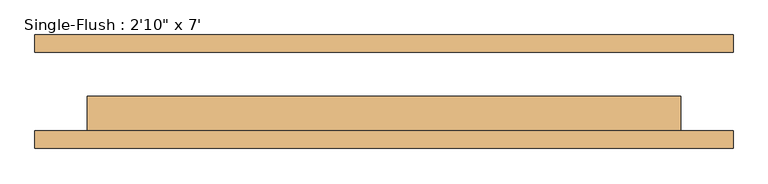
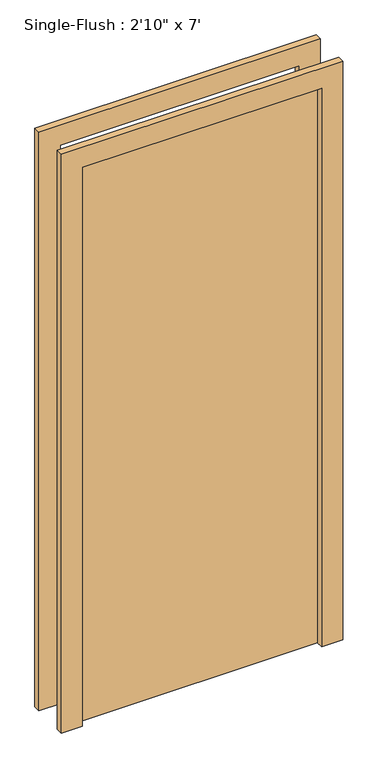
"""IFC4 building model written with IfcOpenShell, lengths in millimetres: door geometry."""

from ifc_helpers import new_model, si_unit, frame, origin, origin_with_axes, place, context, project, spatial, polyline, outline, extrude, source, transform, mapped, element, save


def door_700d3439(model_context):
    return source(origin(), model_context, "Body", "SweptSolid", [
        extrude(outline(polyline([(2209.8, -508.0), (0.0, -508.0), (0.0, -431.8), (2133.6, -431.8), (2133.6, 431.8), (0.0, 431.8), (0.0, 508.0), (2209.8, 508.0), (2209.8, -508.0)])), frame((0.0, -82.55, 0.0), z_axis=(0.0, 1.0, 0.0), x_axis=(0.0, 0.0, 1.0)), (0.0, 0.0, 1.0), 25.4),
        extrude(outline(polyline([(2209.8, 508.0), (2209.8, -508.0), (0.0, -508.0), (0.0, -431.8), (2133.6, -431.8), (2133.6, 431.8), (0.0, 431.8), (0.0, 508.0), (2209.8, 508.0)])), frame((0.0, 57.15, 0.0), z_axis=(0.0, 1.0, 0.0), x_axis=(0.0, 0.0, 1.0)), (0.0, 0.0, 1.0), 25.4),
        extrude(outline(polyline([(431.8, -6.35), (431.8, -57.15), (-431.8, -57.15), (-431.8, -6.35), (431.8, -6.35)])), origin_with_axes(), (0.0, 0.0, 1.0), 2133.6),
    ])


if __name__ == "__main__":
    model = new_model("IFC4")
    model_context = context("Model", 3, world=origin())
    ifc_project = project(units=[si_unit("LENGTHUNIT", "METRE", prefix="MILLI")], contexts=[model_context])
    site = spatial("IfcSite", under=ifc_project)
    building = spatial("IfcBuilding", under=site)
    placement = place(None, origin())
    door_shape = door_700d3439(model_context)
    element("IfcDoor", 1, ObjectType="Single-Flush : 2'10\" x 7'", at=placement, inside=building, context=model_context, shape_type="MappedRepresentation", body=[
        mapped(door_shape, transform((0.0, 0.0, 0.0), x_axis=(1.0, 0.0, 0.0), y_axis=(0.0, 1.0, 0.0), z_axis=(0.0, 0.0, 1.0))),
    ])
    save(model, "model.ifc")

# Revit data of these elements
# Type "Single-Flush : 2'10\" x 7'"
#   Type Mark = "13"
#   Construction Type Id = "MDOOR"
#   Assembly Code = "C1020"
#   Analytic Construction = "Metal"
#   Thickness = 0' - 2"
#   Heat Transfer Coefficient (U) = 0.651978 BTU/(h·ft²·°F)
#   Height = 7' - 0"
#   Trim Projection Ext = 0' - 1"
#   Trim Projection Int = 0' - 1"
#   Trim Width = 0' - 3"
#   Width = 2' - 10"
#   Define Thermal Properties by = 1
#   Door Material = Door - Panel
#   Frame Material = Door - Frame
#   Visual Light Transmittance = 0
#   Solar Heat Gain Coefficient = 0
#   Function = (empty or 0)
#   Wall Closure = (empty or 0)
# Element 1 (IfcDoor, "Single-Flush : 2'10\" x 7'")
#   Materials on its faces: "Door - Frame", "Door - Panel"
# Materials
#   "Door - Panel": class "Wood", colour RGB 210 159 95, transparency 0, Cost = 0
#   "Door - Frame": colour RGB 118 70 51, transparency 0, Cost = 0
